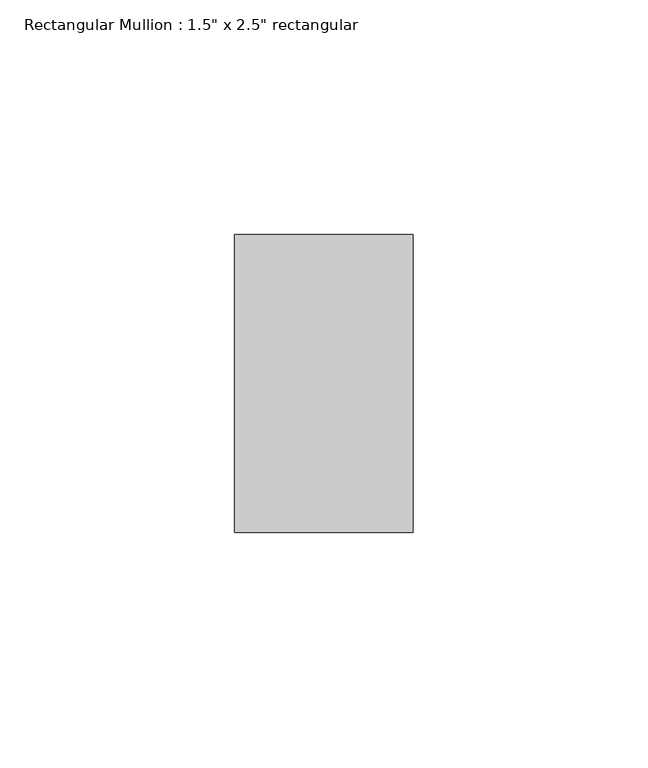
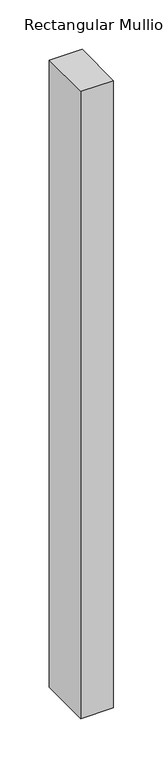
"""IFC4 building model written with IfcOpenShell, lengths in millimetres: member geometry."""

from ifc_helpers import new_model, si_unit, frame, origin, place, context, project, spatial, polyline, outline, extrude, source, transform, mapped, element, save


def member_0748a5fc(model_context):
    return source(origin(), model_context, "Body", "SweptSolid", [
        extrude(outline(polyline([(0.0, 31.75), (0.0, -31.75), (-38.1, -31.75), (-38.1, 31.75), (0.0, 31.75)])), frame((0.0, 0.0, -774.7), z_axis=(0.0, 0.0, 1.0), x_axis=(1.0, 0.0, 0.0)), (0.0, 0.0, 1.0), 774.7),
    ])


if __name__ == "__main__":
    model = new_model("IFC4")
    model_context = context("Model", 3, world=origin())
    ifc_project = project(units=[si_unit("LENGTHUNIT", "METRE", prefix="MILLI")], contexts=[model_context])
    site = spatial("IfcSite", under=ifc_project)
    building = spatial("IfcBuilding", under=site)
    placement = place(None, origin())
    member_shape = member_0748a5fc(model_context)
    element("IfcMember", 1, ObjectType="Rectangular Mullion : 1.5\" x 2.5\" rectangular", at=placement, inside=building, context=model_context, shape_type="MappedRepresentation", body=[
        mapped(member_shape, transform((0.0, 0.0, 0.0), x_axis=(1.0, 0.0, 0.0), y_axis=(0.0, 1.0, 0.0), z_axis=(0.0, 0.0, 1.0))),
    ])
    save(model, "model.ifc")

# Revit data of these elements
# Type "Rectangular Mullion : 1.5\" x 2.5\" rectangular"
#   built-in parameter 1007304 = 0.208333 (stored number, unit not read)
#   built-in parameter 1007301 = 0.0625 (stored number, unit not read)
#   built-in parameter 1007300 = 0.0625 (stored number, unit not read)
# Element 1 (IfcMember, "Rectangular Mullion : 1.5\" x 2.5\" rectangular")
#   Materials on its faces: "Leather - Black"
# Materials
#   "Leather - Black": class "Generic", colour RGB 40 40 40, transparency 0, Cost = 0
